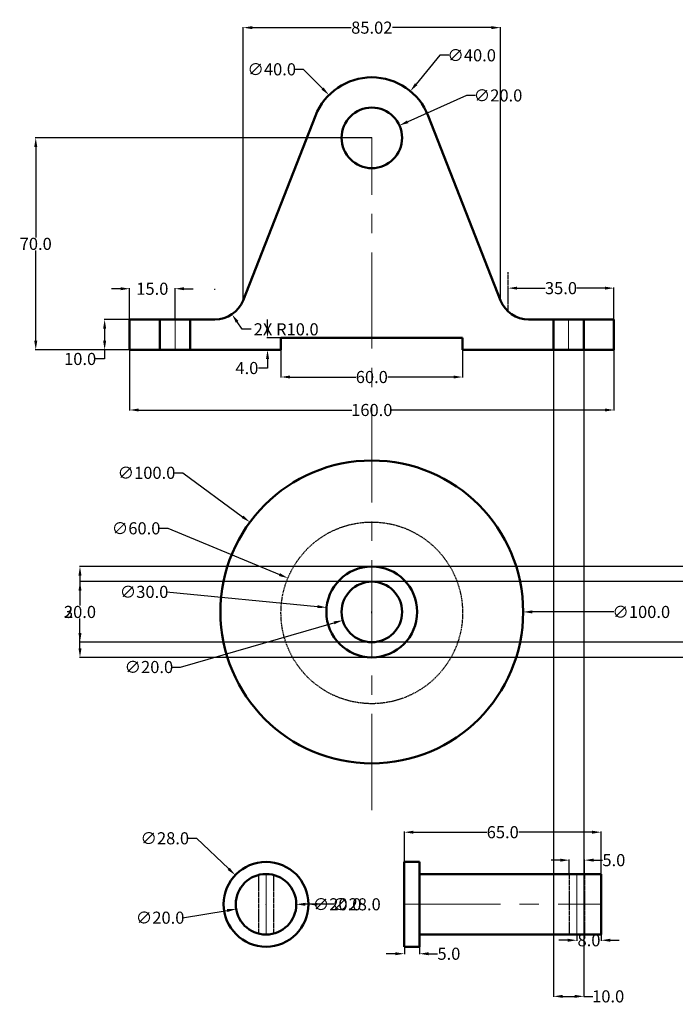
# Model space of a CAD drawing. Units: inches. Extents: x 639 to 969, y 329 to 654.
# Tile 1 of 2: x 639 to 856, y 329 to 654. Entities that reach past the tile are written whole.
import ezdxf

# ---------------------------------------------------------------- set-up
doc = ezdxf.new("R2010")
doc.units = ezdxf.units.IN
doc.header["$MEASUREMENT"] = 0
doc.linetypes.add('CENTER', pattern=[50.8, 31.75, -6.35, 6.35, -6.35])
doc.linetypes.add('HIDDEN', pattern=[0.375, 0.25, -0.125])
for name, color, linetype, lineweight in [('M-CNTR', 1, 'CENTER', 18), ('M-DIMS', 3, 'Continuous', 25), ('M-HIDN', 2, 'HIDDEN', 25), ('M-OUTL', 7, 'Continuous', 50)]:
    doc.layers.add(name, color=color, linetype=linetype, lineweight=lineweight)
doc.styles.get("Standard").update_dxf_attribs({"font": 'arial.ttf'})
doc.dimstyles.get("Standard").update_dxf_attribs({"dimtxt": 4, "dimasz": 3, "dimexe": 0.18, "dimexo": 0.0625, "dimgap": 0.09, "dimtad": 0, "dimtih": 1, "dimtoh": 1, "dimdec": 1, "dimzin": 0, "dimdsep": 46, "dimtxsty": 'Standard', "dimcen": 0.09, "dimadec": 0, "dimazin": 0, "dimtfac": 1, "dimtdec": 1, "dimtofl": 0, "dimtmove": 0, "dimatfit": 3, "dimfxl": 1, "dimtolj": 1, "dimtzin": 0, "dimarcsym": 0})

# ---------------------------------------------------------------- blocks, each defined once
blk = doc.blocks.new('*D8')
at = {"layer": 'Defpoints', "color": 0, "transparency": 16777216}
for p in [(675.43, 545.16), (835.43, 545.16), (835.43, 525.3)]:
    blk.add_point(p, dxfattribs=at)
at = {"layer": 'M-DIMS', "color": 0, "lineweight": -2, "transparency": 16777216}
for p, q in [((675.43, 545.09), (675.43, 525.12)), ((835.43, 545.09), (835.43, 525.12)), ((678.43, 525.3), (748.79, 525.3)), ((832.43, 525.3), (762.07, 525.3))]:
    blk.add_line(p, q, dxfattribs=at)
at = {"layer": 'M-DIMS', "color": 0, "transparency": 16777216}
for points in [[(678.43, 525.8), (678.43, 524.8), (675.43, 525.3)], [(832.43, 525.8), (832.43, 524.8), (835.43, 525.3)]]:
    blk.add_solid(points, dxfattribs=at)
at = {"layer": 'M-DIMS', "color": 0, "transparency": 16777216, "insert": (755.43, 525.3), "char_height": 4, "attachment_point": 5}
blk.add_mtext('\\A1;160.0', dxfattribs=at)
blk = doc.blocks.new('*D9')
at = {"layer": 'Defpoints', "color": 0, "transparency": 16777216}
for p in [(725.43, 547.16), (785.43, 549.16), (785.43, 536.19)]:
    blk.add_point(p, dxfattribs=at)
at = {"layer": 'M-DIMS', "color": 0, "lineweight": -2, "transparency": 16777216}
for p, q in [((725.43, 547.09), (725.43, 536.01)), ((785.43, 549.09), (785.43, 536.01)), ((728.43, 536.19), (750.14, 536.19)), ((782.43, 536.19), (760.72, 536.19))]:
    blk.add_line(p, q, dxfattribs=at)
at = {"layer": 'M-DIMS', "color": 0, "transparency": 16777216}
for points in [[(728.43, 536.69), (728.43, 535.69), (725.43, 536.19)], [(782.43, 536.69), (782.43, 535.69), (785.43, 536.19)]]:
    blk.add_solid(points, dxfattribs=at)
at = {"layer": 'M-DIMS', "color": 0, "transparency": 16777216, "insert": (755.43, 536.19), "char_height": 4, "attachment_point": 5}
blk.add_mtext('\\A1;60.0', dxfattribs=at)
blk = doc.blocks.new('*D10')
at = {"layer": 'Defpoints', "color": 0, "transparency": 16777216}
for p in [(675.43, 565.34), (675.43, 555.16), (690.43, 555.16)]:
    blk.add_point(p, dxfattribs=at)
at = {"layer": 'M-DIMS', "color": 0, "lineweight": -2, "transparency": 16777216}
for p, q in [((672.43, 565.34), (669.43, 565.34)), ((675.43, 555.22), (675.43, 565.52)), ((690.43, 555.22), (690.43, 565.52)), ((693.43, 565.34), (696.43, 565.34))]:
    blk.add_line(p, q, dxfattribs=at)
at = {"layer": 'M-DIMS', "color": 0, "transparency": 16777216}
for points in [[(672.43, 565.84), (672.43, 564.84), (675.43, 565.34)], [(693.43, 565.84), (693.43, 564.84), (690.43, 565.34)]]:
    blk.add_solid(points, dxfattribs=at)
at = {"layer": 'M-DIMS', "color": 0, "transparency": 16777216, "insert": (682.93, 565.34), "char_height": 4, "attachment_point": 5}
blk.add_mtext('\\A1;15.0', dxfattribs=at)
blk = doc.blocks.new('*D11')
at = {"layer": 'Defpoints', "color": 0, "transparency": 16777216}
for p in [(675.47, 555.16), (667.17, 545.16), (674.28, 545.16)]:
    blk.add_point(p, dxfattribs=at)
at = {"layer": 'M-DIMS', "color": 0, "lineweight": -2, "transparency": 16777216}
for p, q in [((675.41, 555.16), (666.99, 555.16)), ((667.17, 552.16), (667.17, 548.16)), ((674.22, 545.16), (666.99, 545.16)), ((667.17, 545.16), (667.17, 542.16)), ((667.17, 542.16), (664.17, 542.16))]:
    blk.add_line(p, q, dxfattribs=at)
at = {"layer": 'M-DIMS', "color": 0, "transparency": 16777216}
for points in [[(666.67, 552.16), (667.67, 552.16), (667.17, 555.16)], [(666.67, 548.16), (667.67, 548.16), (667.17, 545.16)]]:
    blk.add_solid(points, dxfattribs=at)
at = {"layer": 'M-DIMS', "color": 0, "transparency": 16777216, "insert": (659.08, 542.16), "char_height": 4, "attachment_point": 5}
blk.add_mtext('\\A1;10.0', dxfattribs=at)
blk = doc.blocks.new('*D12')
at = {"layer": 'Defpoints', "color": 0, "transparency": 16777216}
for p in [(725.43, 549.16), (720.98, 545.16), (725.43, 545.16)]:
    blk.add_point(p, dxfattribs=at)
at = {"layer": 'M-DIMS', "color": 0, "lineweight": -2, "transparency": 16777216}
for p, q in [((720.98, 552.16), (720.98, 555.16)), ((725.37, 549.16), (720.8, 549.16)), ((725.37, 545.16), (720.8, 545.16)), ((720.98, 542.16), (720.98, 539.16)), ((720.98, 539.16), (717.98, 539.16))]:
    blk.add_line(p, q, dxfattribs=at)
at = {"layer": 'M-DIMS', "color": 0, "transparency": 16777216}
for points in [[(720.48, 552.16), (721.48, 552.16), (720.98, 549.16)], [(720.48, 542.16), (721.48, 542.16), (720.98, 545.16)]]:
    blk.add_solid(points, dxfattribs=at)
at = {"layer": 'M-DIMS', "color": 0, "transparency": 16777216, "insert": (714.17, 539.16), "char_height": 4, "attachment_point": 5}
blk.add_mtext('\\A1;4.0', dxfattribs=at)
blk = doc.blocks.new('*D13')
at = {"layer": 'Defpoints', "color": 0, "transparency": 16777216}
for p in [(768.17, 630.58), (742.69, 599.74)]:
    blk.add_point(p, dxfattribs=at)
at = {"layer": 'M-DIMS', "color": 0, "lineweight": -2, "transparency": 16777216}
for p, q in [((777.95, 642.43), (770.08, 632.89)), ((780.95, 642.43), (777.95, 642.43)), ((755.34, 615.16), (755.52, 615.16)), ((755.43, 615.07), (755.43, 615.25))]:
    blk.add_line(p, q, dxfattribs=at)
at = {"layer": 'M-DIMS', "color": 0, "transparency": 16777216}
blk.add_solid([(769.69, 633.21), (770.46, 632.57), (768.17, 630.58)], dxfattribs=at)
at = {"layer": 'M-DIMS', "color": 0, "transparency": 16777216, "insert": (788.41, 642.43), "char_height": 4, "attachment_point": 5}
blk.add_mtext('\\A1;∅40.0', dxfattribs=at)
blk = doc.blocks.new('*D14')
at = {"layer": 'Defpoints', "color": 0, "transparency": 16777216}
for p in [(764.55, 619.25), (746.3, 611.06)]:
    blk.add_point(p, dxfattribs=at)
at = {"layer": 'M-DIMS', "color": 0, "lineweight": -2, "transparency": 16777216}
for p, q in [((786.68, 629.17), (767.29, 620.48)), ((789.68, 629.17), (786.68, 629.17)), ((755.34, 615.16), (755.52, 615.16)), ((755.43, 615.07), (755.43, 615.25))]:
    blk.add_line(p, q, dxfattribs=at)
at = {"layer": 'M-DIMS', "color": 0, "transparency": 16777216}
blk.add_solid([(767.09, 620.93), (767.5, 620.02), (764.55, 619.25)], dxfattribs=at)
at = {"layer": 'M-DIMS', "color": 0, "transparency": 16777216, "insert": (797.13, 629.17), "char_height": 4, "attachment_point": 5}
blk.add_mtext('\\A1;∅20.0', dxfattribs=at)
blk = doc.blocks.new('*D15')
at = {"layer": 'Defpoints', "color": 0, "transparency": 16777216}
for p in [(715.16, 488.25), (795.7, 428.99)]:
    blk.add_point(p, dxfattribs=at)
at = {"layer": 'M-DIMS', "color": 0, "lineweight": -2, "transparency": 16777216}
for p, q in [((690, 504.56), (693, 504.56)), ((693, 504.56), (712.74, 490.03)), ((755.34, 458.62), (755.52, 458.62)), ((755.43, 458.53), (755.43, 458.71))]:
    blk.add_line(p, q, dxfattribs=at)
at = {"layer": 'M-DIMS', "color": 0, "transparency": 16777216}
blk.add_solid([(713.04, 490.43), (712.44, 489.63), (715.16, 488.25)], dxfattribs=at)
at = {"layer": 'M-DIMS', "color": 0, "transparency": 16777216, "insert": (680.99, 504.56), "char_height": 4, "attachment_point": 5}
blk.add_mtext('\\A1;∅100.0', dxfattribs=at)
blk = doc.blocks.new('*D16')
at = {"layer": 'Defpoints', "color": 0, "transparency": 16777216}
for p in [(727.71, 469.79), (783.14, 446.83)]:
    blk.add_point(p, dxfattribs=at)
at = {"layer": 'M-DIMS', "color": 0, "lineweight": -2, "transparency": 16777216}
for p, q in [((685.03, 486.23), (688.03, 486.23)), ((688.03, 486.23), (724.94, 470.94)), ((755.34, 458.31), (755.52, 458.31)), ((755.43, 458.22), (755.43, 458.4))]:
    blk.add_line(p, q, dxfattribs=at)
at = {"layer": 'M-DIMS', "color": 0, "transparency": 16777216}
blk.add_solid([(725.13, 471.4), (724.75, 470.48), (727.71, 469.79)], dxfattribs=at)
at = {"layer": 'M-DIMS', "color": 0, "transparency": 16777216, "insert": (677.57, 486.23), "char_height": 4, "attachment_point": 5}
blk.add_mtext('\\A1;∅60.0', dxfattribs=at)
blk = doc.blocks.new('*D17')
at = {"layer": 'Defpoints', "color": 0, "transparency": 16777216}
for p in [(740.5, 460.08), (770.36, 457.16)]:
    blk.add_point(p, dxfattribs=at)
at = {"layer": 'M-DIMS', "color": 0, "lineweight": -2, "transparency": 16777216}
for p, q in [((687.65, 465.24), (737.51, 460.37)), ((755.34, 458.62), (755.52, 458.62)), ((755.43, 458.53), (755.43, 458.71))]:
    blk.add_line(p, q, dxfattribs=at)
at = {"layer": 'M-DIMS', "color": 0, "transparency": 16777216}
blk.add_solid([(737.56, 460.87), (737.47, 459.87), (740.5, 460.08)], dxfattribs=at)
at = {"layer": 'M-DIMS', "color": 0, "transparency": 16777216, "insert": (680.19, 465.24), "char_height": 4, "attachment_point": 5}
blk.add_mtext('\\A1;∅30.0', dxfattribs=at)
blk = doc.blocks.new('*D18')
at = {"layer": 'Defpoints', "color": 0, "transparency": 16777216}
for p in [(765.04, 461.39), (745.82, 455.85)]:
    blk.add_point(p, dxfattribs=at)
at = {"layer": 'M-DIMS', "color": 0, "lineweight": -2, "transparency": 16777216}
for p, q in [((755.34, 458.62), (755.52, 458.62)), ((755.43, 458.53), (755.43, 458.71)), ((692.23, 440.43), (742.94, 455.02)), ((689.23, 440.43), (692.23, 440.43))]:
    blk.add_line(p, q, dxfattribs=at)
at = {"layer": 'M-DIMS', "color": 0, "transparency": 16777216}
blk.add_solid([(742.8, 455.5), (743.07, 454.54), (745.82, 455.85)], dxfattribs=at)
at = {"layer": 'M-DIMS', "color": 0, "transparency": 16777216, "insert": (681.78, 440.43), "char_height": 4, "attachment_point": 5}
blk.add_mtext('\\A1;∅20.0', dxfattribs=at)
blk = doc.blocks.new('*D19')
at = {"layer": 'Defpoints', "color": 0, "transparency": 16777216}
for p in [(710.33, 371.71), (730.65, 352.45)]:
    blk.add_point(p, dxfattribs=at)
at = {"layer": 'M-DIMS', "color": 0, "lineweight": -2, "transparency": 16777216}
for p, q in [((694.49, 383.88), (697.49, 383.88)), ((697.49, 383.88), (708.15, 373.78)), ((720.4, 362.08), (720.58, 362.08)), ((720.49, 361.99), (720.49, 362.17))]:
    blk.add_line(p, q, dxfattribs=at)
at = {"layer": 'M-DIMS', "color": 0, "transparency": 16777216}
blk.add_solid([(708.5, 374.14), (707.81, 373.42), (710.33, 371.71)], dxfattribs=at)
at = {"layer": 'M-DIMS', "color": 0, "transparency": 16777216, "insert": (687.04, 383.88), "char_height": 4, "attachment_point": 5}
blk.add_mtext('\\A1;∅28.0', dxfattribs=at)
blk = doc.blocks.new('*D20')
at = {"layer": 'Defpoints', "color": 0, "transparency": 16777216}
for p in [(730.37, 363.67), (710.62, 360.5)]:
    blk.add_point(p, dxfattribs=at)
at = {"layer": 'M-DIMS', "color": 0, "lineweight": -2, "transparency": 16777216}
for p, q in [((720.4, 362.08), (720.58, 362.08)), ((720.49, 361.99), (720.49, 362.17)), ((692.95, 357.66), (707.66, 360.02))]:
    blk.add_line(p, q, dxfattribs=at)
at = {"layer": 'M-DIMS', "color": 0, "transparency": 16777216}
blk.add_solid([(707.58, 360.52), (707.74, 359.53), (710.62, 360.5)], dxfattribs=at)
at = {"layer": 'M-DIMS', "color": 0, "transparency": 16777216, "insert": (685.5, 357.66), "char_height": 4, "attachment_point": 5}
blk.add_mtext('\\A1;∅20.0', dxfattribs=at)
blk = doc.blocks.new('*D21')
at = {"layer": 'Defpoints', "color": 0, "transparency": 16777216}
for p in [(825.68, 376.66), (820.68, 372.08), (825.68, 372.08)]:
    blk.add_point(p, dxfattribs=at)
at = {"layer": 'M-DIMS', "color": 0, "lineweight": -2, "transparency": 16777216}
for p, q in [((817.68, 376.66), (814.68, 376.66)), ((820.68, 372.15), (820.68, 376.84)), ((825.68, 372.15), (825.68, 376.84)), ((828.68, 376.66), (831.68, 376.66))]:
    blk.add_line(p, q, dxfattribs=at)
at = {"layer": 'M-DIMS', "color": 0, "transparency": 16777216}
for points in [[(817.68, 377.16), (817.68, 376.16), (820.68, 376.66)], [(828.68, 377.16), (828.68, 376.16), (825.68, 376.66)]]:
    blk.add_solid(points, dxfattribs=at)
at = {"layer": 'M-DIMS', "color": 0, "transparency": 16777216, "insert": (835.4, 376.66), "char_height": 4, "attachment_point": 5}
blk.add_mtext('\\A1;5.0', dxfattribs=at)
blk = doc.blocks.new('*D22')
at = {"layer": 'Defpoints', "color": 0, "transparency": 16777216}
for p in [(766.18, 348.08), (771.18, 348.08), (771.18, 345.76)]:
    blk.add_point(p, dxfattribs=at)
at = {"layer": 'M-DIMS', "color": 0, "lineweight": -2, "transparency": 16777216}
for p, q in [((766.18, 348.02), (766.18, 345.58)), ((771.18, 348.02), (771.18, 345.58)), ((763.18, 345.76), (760.18, 345.76)), ((774.18, 345.76), (777.18, 345.76))]:
    blk.add_line(p, q, dxfattribs=at)
at = {"layer": 'M-DIMS', "color": 0, "transparency": 16777216}
for points in [[(763.18, 346.26), (763.18, 345.26), (766.18, 345.76)], [(774.18, 346.26), (774.18, 345.26), (771.18, 345.76)]]:
    blk.add_solid(points, dxfattribs=at)
at = {"layer": 'M-DIMS', "color": 0, "transparency": 16777216, "insert": (780.9, 345.76), "char_height": 4, "attachment_point": 5}
blk.add_mtext('\\A1;5.0', dxfattribs=at)
blk = doc.blocks.new('*D23')
at = {"layer": 'Defpoints', "color": 0, "transparency": 16777216}
for p in [(823.18, 352.08), (831.18, 352.08), (831.18, 350.21)]:
    blk.add_point(p, dxfattribs=at)
at = {"layer": 'M-DIMS', "color": 0, "lineweight": -2, "transparency": 16777216}
for p, q in [((823.18, 352.02), (823.18, 350.03)), ((831.18, 352.02), (831.18, 350.03)), ((820.18, 350.21), (817.18, 350.21)), ((834.18, 350.21), (837.18, 350.21))]:
    blk.add_line(p, q, dxfattribs=at)
at = {"layer": 'M-DIMS', "color": 0, "transparency": 16777216}
for points in [[(820.18, 350.71), (820.18, 349.71), (823.18, 350.21)], [(834.18, 350.71), (834.18, 349.71), (831.18, 350.21)]]:
    blk.add_solid(points, dxfattribs=at)
at = {"layer": 'M-DIMS', "color": 0, "transparency": 16777216, "insert": (827.18, 350.21), "char_height": 4, "attachment_point": 5}
blk.add_mtext('\\A1;8.0', dxfattribs=at)
blk = doc.blocks.new('*D24')
at = {"layer": 'Defpoints', "color": 0, "transparency": 16777216}
for p in [(831.18, 385.89), (766.18, 376.08), (831.18, 372.08)]:
    blk.add_point(p, dxfattribs=at)
at = {"layer": 'M-DIMS', "color": 0, "lineweight": -2, "transparency": 16777216}
for p, q in [((766.18, 376.15), (766.18, 386.07)), ((769.18, 385.89), (793.39, 385.89)), ((828.18, 385.89), (803.97, 385.89)), ((831.18, 372.15), (831.18, 386.07))]:
    blk.add_line(p, q, dxfattribs=at)
at = {"layer": 'M-DIMS', "color": 0, "transparency": 16777216}
for points in [[(769.18, 386.39), (769.18, 385.39), (766.18, 385.89)], [(828.18, 386.39), (828.18, 385.39), (831.18, 385.89)]]:
    blk.add_solid(points, dxfattribs=at)
at = {"layer": 'M-DIMS', "color": 0, "transparency": 16777216, "insert": (798.68, 385.89), "char_height": 4, "attachment_point": 5}
blk.add_mtext('\\A1;65.0', dxfattribs=at)
blk = doc.blocks.new('*D25')
at = {"layer": 'Defpoints', "color": 0, "transparency": 16777216}
for p in [(755.52, 615.16), (644.41, 545.16), (725.43, 545.16)]:
    blk.add_point(p, dxfattribs=at)
at = {"layer": 'M-DIMS', "color": 0, "lineweight": -2, "transparency": 16777216}
for p, q in [((755.46, 615.16), (644.23, 615.16)), ((644.41, 612.16), (644.41, 582.29)), ((644.41, 548.16), (644.41, 578.02)), ((725.37, 545.16), (644.23, 545.16))]:
    blk.add_line(p, q, dxfattribs=at)
at = {"layer": 'M-DIMS', "color": 0, "transparency": 16777216}
for points in [[(643.91, 612.16), (644.91, 612.16), (644.41, 615.16)], [(643.91, 548.16), (644.91, 548.16), (644.41, 545.16)]]:
    blk.add_solid(points, dxfattribs=at)
at = {"layer": 'M-DIMS', "color": 0, "transparency": 16777216, "insert": (644.41, 580.16), "char_height": 4, "attachment_point": 5}
blk.add_mtext('\\A1;70.0', dxfattribs=at)
blk = doc.blocks.new('*D29')
at = {"layer": 'Defpoints', "color": 0, "transparency": 16777216}
for p in [(800.43, 564.35), (835.43, 565.54), (835.43, 555.16)]:
    blk.add_point(p, dxfattribs=at)
at = {"layer": 'M-DIMS', "color": 0, "lineweight": -2, "transparency": 16777216}
for p, q in [((800.43, 564.42), (800.43, 565.72)), ((835.43, 555.22), (835.43, 565.72)), ((803.43, 565.54), (812.65, 565.54)), ((832.43, 565.54), (823.21, 565.54))]:
    blk.add_line(p, q, dxfattribs=at)
at = {"layer": 'M-DIMS', "color": 0, "transparency": 16777216}
for points in [[(803.43, 566.04), (803.43, 565.04), (800.43, 565.54)], [(832.43, 566.04), (832.43, 565.04), (835.43, 565.54)]]:
    blk.add_solid(points, dxfattribs=at)
at = {"layer": 'M-DIMS', "color": 0, "transparency": 16777216, "insert": (817.93, 565.54), "char_height": 4, "attachment_point": 5}
blk.add_mtext('\\A1;35.0', dxfattribs=at)
blk = doc.blocks.new('*D30')
at = {"layer": 'Defpoints', "color": 0, "transparency": 16777216}
for p in [(815.429038, 545.157004), (825.429038, 545.157004), (825.429038, 331.683003)]:
    blk.add_point(p, dxfattribs=at)
at = {"layer": 'M-DIMS', "color": 0, "lineweight": -2, "transparency": 16777216}
for p, q in [((815.429038, 545.094504), (815.429038, 331.503003)), ((825.429038, 545.094504), (825.429038, 331.503003)), ((818.429038, 331.683003), (822.429038, 331.683003)), ((825.429038, 331.683003), (828.429038, 331.683003))]:
    blk.add_line(p, q, dxfattribs=at)
at = {"layer": 'M-DIMS', "color": 0, "transparency": 16777216}
for points in [[(818.429038, 332.183003), (818.429038, 331.183003), (815.429038, 331.683003)], [(822.429038, 332.183003), (822.429038, 331.183003), (825.429038, 331.683003)]]:
    blk.add_solid(points, dxfattribs=at)
at = {"layer": 'M-DIMS', "color": 0, "transparency": 16777216, "insert": (833.519038, 331.683003), "char_height": 4, "attachment_point": 5}
blk.add_mtext('\\A1;10.0', dxfattribs=at)
blk = doc.blocks.new('*D31')
at = {"layer": 'Defpoints', "color": 0, "transparency": 16777216}
for p in [(797.94, 651.56), (712.92, 561.51), (797.94, 561.51)]:
    blk.add_point(p, dxfattribs=at)
at = {"layer": 'M-DIMS', "color": 0, "lineweight": -2, "transparency": 16777216}
for p, q in [((712.92, 561.57), (712.92, 651.74)), ((715.92, 651.56), (748.61, 651.56)), ((794.94, 651.56), (762.25, 651.56)), ((797.94, 561.57), (797.94, 651.74))]:
    blk.add_line(p, q, dxfattribs=at)
at = {"layer": 'M-DIMS', "color": 0, "transparency": 16777216}
for points in [[(715.92, 652.06), (715.92, 651.06), (712.92, 651.56)], [(794.94, 652.06), (794.94, 651.06), (797.94, 651.56)]]:
    blk.add_solid(points, dxfattribs=at)
at = {"layer": 'M-DIMS', "color": 0, "transparency": 16777216, "insert": (755.43, 651.56), "char_height": 4, "attachment_point": 5}
blk.add_mtext('\\A1;85.02', dxfattribs=at)
blk = doc.blocks.new('*D34')
at = {"layer": 'Defpoints', "color": 0, "transparency": 16777216}
for p in [(659.03, 473.62), (896.74, 473.62), (896.74, 443.62)]:
    blk.add_point(p, dxfattribs=at)
at = {"layer": 'M-DIMS', "color": 0, "lineweight": -2, "transparency": 16777216}
for p, q in [((896.67, 473.62), (658.85, 473.62)), ((659.03, 470.62), (659.03, 460.75)), ((659.03, 446.62), (659.03, 456.49)), ((896.67, 443.62), (658.85, 443.62))]:
    blk.add_line(p, q, dxfattribs=at)
at = {"layer": 'M-DIMS', "color": 0, "transparency": 16777216}
for points in [[(658.53, 470.62), (659.53, 470.62), (659.03, 473.62)], [(658.53, 446.62), (659.53, 446.62), (659.03, 443.62)]]:
    blk.add_solid(points, dxfattribs=at)
at = {"layer": 'M-DIMS', "color": 0, "transparency": 16777216, "insert": (659.03, 458.62), "char_height": 4, "attachment_point": 5}
blk.add_mtext('\\A1;30.0', dxfattribs=at)
blk = doc.blocks.new('*D35')
at = {"layer": 'Defpoints', "color": 0, "transparency": 16777216}
for p in [(659.03, 468.62), (898.74, 468.62), (898.74, 448.62)]:
    blk.add_point(p, dxfattribs=at)
at = {"layer": 'M-DIMS', "color": 0, "lineweight": -2, "transparency": 16777216}
for p, q in [((898.67, 468.62), (658.85, 468.62)), ((659.03, 465.62), (659.03, 460.75)), ((659.03, 451.62), (659.03, 456.49)), ((898.67, 448.62), (658.85, 448.62))]:
    blk.add_line(p, q, dxfattribs=at)
at = {"layer": 'M-DIMS', "color": 0, "transparency": 16777216}
for points in [[(658.53, 465.62), (659.53, 465.62), (659.03, 468.62)], [(658.53, 451.62), (659.53, 451.62), (659.03, 448.62)]]:
    blk.add_solid(points, dxfattribs=at)
at = {"layer": 'M-DIMS', "color": 0, "transparency": 16777216, "insert": (659.03, 458.62), "char_height": 4, "attachment_point": 5}
blk.add_mtext('\\A1;20.0', dxfattribs=at)
blk = doc.blocks.new('*D36')
at = {"layer": 'Defpoints', "color": 0, "transparency": 16777216}
for p in [(703.61, 565.16), (709.24, 556.9)]:
    blk.add_point(p, dxfattribs=at)
at = {"layer": 'M-DIMS', "color": 0, "lineweight": -2, "transparency": 16777216}
for p, q in [((703.52, 565.16), (703.7, 565.16)), ((703.61, 565.07), (703.61, 565.25)), ((712.62, 551.94), (710.93, 554.42)), ((715.62, 551.94), (712.62, 551.94))]:
    blk.add_line(p, q, dxfattribs=at)
at = {"layer": 'M-DIMS', "color": 0, "transparency": 16777216}
blk.add_solid([(711.35, 554.7), (710.52, 554.14), (709.24, 556.9)], dxfattribs=at)
at = {"layer": 'M-DIMS', "color": 0, "transparency": 16777216, "insert": (727.15, 551.94), "char_height": 4, "attachment_point": 5}
blk.add_mtext('\\A1;2X R10.0', dxfattribs=at)
blk = doc.blocks.new('*D38')
at = {"layer": 'Defpoints', "color": 0, "transparency": 16777216}
for p in [(741.29, 629.31), (769.56, 601.01)]:
    blk.add_point(p, dxfattribs=at)
at = {"layer": 'M-DIMS', "color": 0, "lineweight": -2, "transparency": 16777216}
for p, q in [((729.81, 637.8), (732.81, 637.8)), ((732.81, 637.8), (739.17, 631.43)), ((755.34, 615.16), (755.52, 615.16)), ((755.43, 615.07), (755.43, 615.25))]:
    blk.add_line(p, q, dxfattribs=at)
at = {"layer": 'M-DIMS', "color": 0, "transparency": 16777216}
blk.add_solid([(739.53, 631.78), (738.82, 631.08), (741.29, 629.31)], dxfattribs=at)
at = {"layer": 'M-DIMS', "color": 0, "transparency": 16777216, "insert": (722.36, 637.8), "char_height": 4, "attachment_point": 5}
blk.add_mtext('\\A1;∅40.0', dxfattribs=at)
blk = doc.blocks.new('*D39')
at = {"layer": 'Defpoints', "color": 0, "transparency": 16777216}
for p in [(705.43, 458.62), (805.43, 458.62)]:
    blk.add_point(p, dxfattribs=at)
at = {"layer": 'M-DIMS', "color": 0, "lineweight": -2, "transparency": 16777216}
for p, q in [((755.34, 458.62), (755.52, 458.62)), ((755.43, 458.53), (755.43, 458.71)), ((835.43, 458.62), (808.43, 458.62))]:
    blk.add_line(p, q, dxfattribs=at)
at = {"layer": 'M-DIMS', "color": 0, "transparency": 16777216}
blk.add_solid([(808.43, 459.12), (808.43, 458.12), (805.43, 458.62)], dxfattribs=at)
at = {"layer": 'M-DIMS', "color": 0, "transparency": 16777216, "insert": (844.44, 458.62), "char_height": 4, "attachment_point": 5}
blk.add_mtext('\\A1;∅100.0', dxfattribs=at)
blk = doc.blocks.new('*D40')
at = {"layer": 'Defpoints', "color": 0, "transparency": 16777216}
for p in [(706.49, 362.08), (734.49, 362.08)]:
    blk.add_point(p, dxfattribs=at)
at = {"layer": 'M-DIMS', "color": 0, "lineweight": -2, "transparency": 16777216}
for p, q in [((720.4, 362.08), (720.58, 362.08)), ((720.49, 361.99), (720.49, 362.17)), ((742.89, 362.08), (737.49, 362.08))]:
    blk.add_line(p, q, dxfattribs=at)
at = {"layer": 'M-DIMS', "color": 0, "transparency": 16777216}
blk.add_solid([(737.49, 362.58), (737.49, 361.58), (734.49, 362.08)], dxfattribs=at)
at = {"layer": 'M-DIMS', "color": 0, "transparency": 16777216, "insert": (750.35, 362.08), "char_height": 4, "attachment_point": 5}
blk.add_mtext('\\A1;∅28.0', dxfattribs=at)
blk = doc.blocks.new('*D41')
at = {"layer": 'Defpoints', "color": 0, "transparency": 16777216}
for p in [(710.49, 362.08), (730.49, 362.08)]:
    blk.add_point(p, dxfattribs=at)
at = {"layer": 'M-DIMS', "color": 0, "lineweight": -2, "transparency": 16777216}
for p, q in [((720.4, 362.08), (720.58, 362.08)), ((720.49, 361.99), (720.49, 362.17)), ((736.49, 362.08), (733.49, 362.08))]:
    blk.add_line(p, q, dxfattribs=at)
at = {"layer": 'M-DIMS', "color": 0, "transparency": 16777216}
blk.add_solid([(733.49, 362.58), (733.49, 361.58), (730.49, 362.08)], dxfattribs=at)
at = {"layer": 'M-DIMS', "color": 0, "transparency": 16777216, "insert": (743.95, 362.08), "char_height": 4, "attachment_point": 5}
blk.add_mtext('\\A1;∅20.0', dxfattribs=at)

msp = doc.modelspace()

# ---------------------------------------------------------------- linework, layer by layer
at = {"layer": 'M-CNTR'}
for p, q in [((755.429, 393.182), (755.429, 615.157)), ((690.429, 555.157), (690.429, 545.157)), ((820.429, 545.157), (820.429, 555.157)), ((720.492, 372.083), (720.492, 352.083)), ((823.177, 372.083), (823.177, 352.083)), ((766.177, 362.083), (831.177, 362.083))]:
    msp.add_line(p, q, dxfattribs=at)
at = {"layer": 'M-HIDN'}
for p, q in [((800.429, 557.844), (800.429, 570.863)), ((717.992, 371.765), (717.992, 352.401)), ((722.992, 371.765), (722.992, 352.401)), ((820.677, 372.083), (820.677, 352.083)), ((825.677, 372.083), (825.677, 352.083))]:
    msp.add_line(p, q, dxfattribs=at)
msp.add_circle((755.429, 458.312), 30, dxfattribs=at)
at = {"layer": 'M-OUTL'}
for p, q in [((736.808, 622.456), (712.918, 561.508)), ((774.05, 622.456), (797.94, 561.508)), ((675.429, 555.157), (675.429, 545.157)), ((703.608, 555.157), (675.429, 555.157)), ((685.429, 555.157), (685.429, 545.157)), ((695.429, 555.157), (695.429, 545.157)), ((835.429, 555.157), (807.25, 555.157)), ((815.429, 545.157), (815.429, 555.157)), ((825.429, 545.157), (825.429, 555.157)), ((835.429, 545.157), (835.429, 555.157)), ((725.429, 545.157), (725.429, 549.157)), ((725.429, 549.157), (785.429, 549.157)), ((785.429, 545.157), (785.429, 549.157)), ((675.429, 545.157), (725.429, 545.157)), ((785.429, 545.157), (835.429, 545.157)), ((766.177, 376.083), (771.177, 376.083)), ((766.177, 376.083), (766.177, 348.083)), ((771.177, 376.083), (771.177, 348.083)), ((771.177, 372.083), (831.177, 372.083)), ((831.177, 372.083), (831.177, 352.083)), ((771.177, 352.083), (831.177, 352.083)), ((766.177, 348.083), (771.177, 348.083))]:
    msp.add_line(p, q, dxfattribs=at)
for centre, radius in [((755.429, 615.157), 10), ((755.429, 458.621), 50), ((755.429, 458.621), 15), ((755.429, 458.621), 10), ((720.492, 362.083), 14), ((720.492, 362.083), 10)]:
    msp.add_circle(centre, radius, dxfattribs=at)
for centre, radius, start, end in [((755.429, 615.157), 20, 21.40389, 158.59611), ((703.608, 565.157), 10, 270, 338.59611), ((807.25, 565.157), 10, 201.40389, 270)]:
    msp.add_arc(centre, radius, start, end, dxfattribs=at)

# ---------------------------------------------------------------- dimensions: what is measured, and where the dimension line sits
at = {"layer": 'M-DIMS'}
for base, p1, p2, override, picture, middle in [((797.94, 651.557), (712.918, 561.508), (797.94, 561.508), {"dimdec": 2, "dimlfac": 1, "dimrnd": 0, "dimzin": 0, "dimdsep": 46, "dimlunit": 2}, '*D31', (755.429, 651.557)), ((675.429, 565.335), (690.429, 555.157), (675.429, 555.157), {"dimclrd": 0, "dimclre": 0, "dimclrt": 0}, '*D10', (682.929, 565.335)), ((835.429, 565.544), (800.429, 564.354), (835.429, 555.157), {"dimclrd": 0, "dimclre": 0, "dimclrt": 0}, '*D29', (817.929, 565.544)), ((785.429, 536.19), (725.429, 547.157), (785.429, 549.157), {"dimclrd": 0, "dimclre": 0, "dimclrt": 0}, '*D9', (755.429, 536.19)), ((835.429, 525.301), (675.429, 545.157), (835.429, 545.157), {"dimclrd": 0, "dimclre": 0, "dimclrt": 0}, '*D8', (755.429, 525.301)), ((825.429, 331.683), (815.429, 545.157), (825.429, 545.157), {"dimdec": 1, "dimlfac": 1, "dimrnd": 0, "dimzin": 0, "dimdsep": 46, "dimlunit": 2}, '*D30', (833.519, 331.683)), ((831.177, 385.89), (766.177, 376.083), (831.177, 372.083), {"dimclrd": 0, "dimclre": 0, "dimclrt": 0}, '*D24', (798.677, 385.89)), ((825.677, 376.658), (820.677, 372.083), (825.677, 372.083), {"dimclrd": 0, "dimclre": 0, "dimclrt": 0}, '*D21', (835.401, 376.658)), ((831.177, 350.209), (823.177, 352.083), (831.177, 352.083), {"dimclrd": 0, "dimclre": 0, "dimclrt": 0}, '*D23', (827.177, 350.209)), ((771.177, 345.764), (766.177, 348.083), (771.177, 348.083), {"dimclrd": 0, "dimclre": 0, "dimclrt": 0}, '*D22', (780.901, 345.764))]:
    dim = msp.add_linear_dim(base=base, p1=p1, p2=p2, dimstyle='Standard', override=override, dxfattribs=at)
    dim.commit()
    dim.dimension.update_dxf_attribs({"geometry": picture, "text_midpoint": middle})
for p1, p2, override, picture, middle in [((742.692, 599.737), (768.166, 630.577), {"dimclrd": 0, "dimclre": 0, "dimclrt": 0}, '*D13', (788.409, 642.426)), ((769.564, 601.008), (741.294, 629.306), {"dimdec": 1, "dimlfac": 1, "dimrnd": 0, "dimzin": 0, "dimdsep": 46, "dimlunit": 2}, '*D38', (722.359, 637.796)), ((746.305, 611.065), (764.553, 619.249), {"dimclrd": 0, "dimclre": 0, "dimclrt": 0}, '*D14', (797.131, 629.17)), ((795.702, 428.989), (715.156, 488.253), {"dimclrd": 0, "dimclre": 0, "dimclrt": 0}, '*D15', (680.989, 504.557)), ((783.145, 446.83), (727.713, 469.793), {"dimclrd": 0, "dimclre": 0, "dimclrt": 0}, '*D16', (677.574, 486.233)), ((770.358, 457.163), (740.5, 460.078), {"dimclrd": 0, "dimclre": 0, "dimclrt": 0}, '*D17', (687.646, 465.238)), ((765.039, 461.387), (745.819, 455.854), {"dimclrd": 0, "dimclre": 0, "dimclrt": 0}, '*D18', (681.778, 440.426)), ((705.429, 458.621), (805.429, 458.62), {"dimdec": 1, "dimlfac": 1, "dimrnd": 0, "dimzin": 0, "dimdsep": 46, "dimlunit": 2}, '*D39', (835.429, 458.62)), ((730.652, 352.451), (710.331, 371.715), {"dimclrd": 0, "dimclre": 0, "dimclrt": 0}, '*D19', (687.04, 383.884)), ((706.492, 362.083), (734.492, 362.083), {"dimdec": 1, "dimlfac": 1, "dimrnd": 0, "dimzin": 0, "dimdsep": 46, "dimlunit": 2}, '*D40', (742.892, 362.083)), ((710.492, 362.083), (730.492, 362.083), {"dimdec": 1, "dimlfac": 1, "dimrnd": 0, "dimzin": 0, "dimdsep": 46, "dimlunit": 2}, '*D41', (736.492, 362.083)), ((730.365, 363.669), (710.618, 360.497), {"dimclrd": 0, "dimclre": 0, "dimclrt": 0}, '*D20', (692.95, 357.659))]:
    dim = msp.add_diameter_dim_2p(p1=p1, p2=p2, dimstyle='Standard', override=override, dxfattribs=at)
    dim.commit()
    dim.dimension.update_dxf_attribs({"geometry": picture, "text_midpoint": middle, "dimtype": 163})
for base, p1, p2, override, picture, middle in [((644.411, 545.157), (755.519, 615.157), (725.429, 545.157), {"dimclrd": 0, "dimclre": 0, "dimclrt": 0}, '*D25', (644.411, 580.157)), ((667.173, 545.157), (675.469, 555.157), (674.284, 545.157), {"dimclrd": 0, "dimclre": 0, "dimclrt": 0}, '*D11', (659.083, 542.157)), ((720.979, 545.157), (725.429, 549.157), (725.429, 545.157), {"dimclrd": 0, "dimclre": 0, "dimclrt": 0}, '*D12', (714.174, 539.157)), ((659.029, 473.621), (896.736, 443.621), (896.736, 473.621), {"dimdec": 1, "dimlfac": 1, "dimrnd": 0, "dimzin": 0, "dimdsep": 46, "dimlunit": 2}, '*D34', (659.029, 458.621)), ((659.029, 468.621), (898.736, 448.621), (898.736, 468.621), {"dimdec": 1, "dimlfac": 1, "dimrnd": 0, "dimzin": 0, "dimdsep": 46, "dimlunit": 2}, '*D35', (659.029, 458.621))]:
    dim = msp.add_linear_dim(base=base, p1=p1, p2=p2, angle=90, dimstyle='Standard', override=override, dxfattribs=at)
    dim.commit()
    dim.dimension.update_dxf_attribs({"geometry": picture, "text_midpoint": middle})
dim = msp.add_radius_dim(center=(703.608, 565.157), mpoint=(709.243, 556.896), text='2X <>', dimstyle='Standard', override={"dimdec": 1, "dimlfac": 1, "dimrnd": 0, "dimzin": 0, "dimdsep": 46, "dimlunit": 2}, dxfattribs=at)
dim.commit()
dim.dimension.update_dxf_attribs({"geometry": '*D36', "text_midpoint": (727.148, 551.939), "dimtype": 164})

doc.saveas('drawing.dxf')
